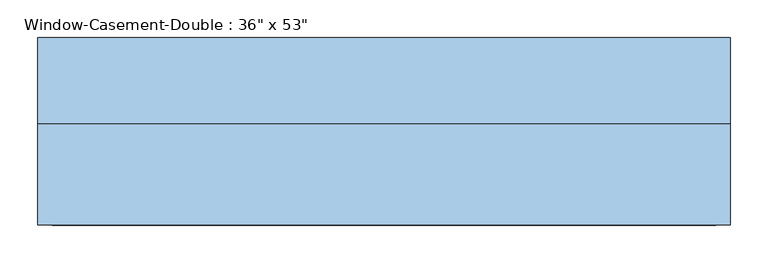
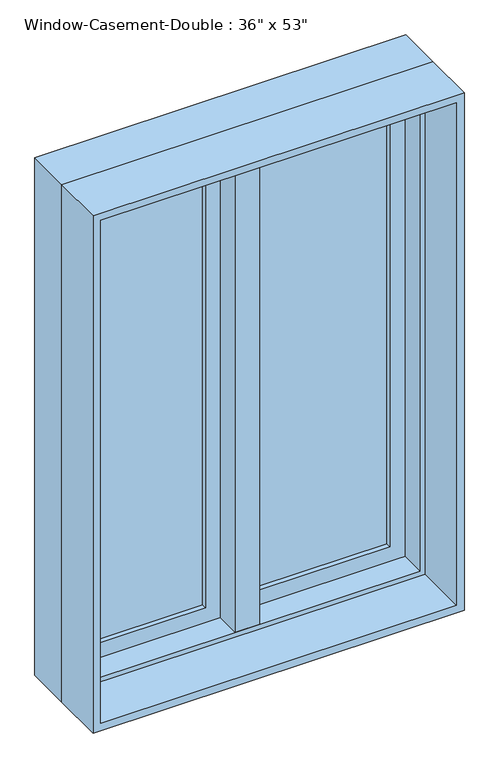
"""IFC4 building model written with IfcOpenShell, lengths in millimetres: window geometry."""

from ifc_helpers import new_model, si_unit, frame, origin, place, context, project, spatial, polyline, outline, extrude, faceted_brep, source, transform, mapped, element, save


def window_79f73a1a(model_context):
    return source(origin(), model_context, "Body", "SolidModel", [
        faceted_brep([(9.525, 133.35, 2247.9), (-9.525, 133.35, 2247.9), (-9.525, 82.55, 2247.9), (9.525, 82.55, 2247.9), (9.525, 133.35, 927.1), (9.525, 82.55, 927.1), (-9.525, 82.55, 927.1), (-9.525, 133.35, 927.1), (-9.525, 82.55, 946.15), (-9.525, 82.55, 2228.85), (-30.1625, 82.55, 946.15), (-30.1625, 82.55, 2228.85), (-30.1625, 19.05, 946.15), (-30.1625, 19.05, 2228.85), (30.1625, 19.05, 946.15), (30.1625, 19.05, 2228.85), (30.1625, 82.55, 946.15), (30.1625, 82.55, 2228.85), (9.525, 82.55, 946.15), (9.525, 82.55, 2228.85)], [[[0, 1, 2, 3]], [[4, 5, 6, 7]], [[1, 0, 4, 7]], [[2, 1, 7, 6, 8, 9]], [[9, 8, 10, 11]], [[11, 10, 12, 13]], [[13, 12, 14, 15]], [[15, 14, 16, 17]], [[17, 16, 18, 19]], [[0, 3, 19, 18, 5, 4]], [[18, 8, 6, 5]], [[9, 19, 3, 2]], [[8, 18, 16, 14, 12, 10]], [[19, 9, 11, 13, 15, 17]]]),
        extrude(outline(polyline([(-66.675, 114.3), (-66.675, 107.95), (-387.35, 107.95), (-387.35, 114.3), (-66.675, 114.3)])), frame((0.0, 0.0, 984.25), z_axis=(0.0, 0.0, 1.0), x_axis=(1.0, 0.0, 0.0)), (0.0, 0.0, 1.0), 1206.5),
        extrude(outline(polyline([(-387.35, 95.25), (-387.35, 101.6), (-66.675, 101.6), (-66.675, 95.25), (-387.35, 95.25)])), frame((0.0, 0.0, 984.25), z_axis=(0.0, 0.0, 1.0), x_axis=(1.0, 0.0, 0.0)), (0.0, 0.0, 1.0), 1206.5),
        extrude(outline(polyline([(387.35, 114.3), (387.35, 107.95), (66.675, 107.95), (66.675, 114.3), (387.35, 114.3)])), frame((0.0, 0.0, 984.25), z_axis=(0.0, 0.0, 1.0), x_axis=(1.0, 0.0, 0.0)), (0.0, 0.0, 1.0), 1206.5),
        extrude(outline(polyline([(66.675, 95.25), (66.675, 101.6), (387.35, 101.6), (387.35, 95.25), (66.675, 95.25)])), frame((0.0, 0.0, 984.25), z_axis=(0.0, 0.0, 1.0), x_axis=(1.0, 0.0, 0.0)), (0.0, 0.0, 1.0), 1206.5),
        extrude(outline(polyline([(2247.9, -444.5), (927.1, -444.5), (927.1, -9.525), (2247.9, -9.525), (2247.9, -444.5)]), holes=[polyline([(2190.75, -66.675), (984.25, -66.675), (984.25, -387.35), (2190.75, -387.35), (2190.75, -66.675)])]), frame((0.0, 82.55, 0.0), z_axis=(0.0, 1.0, 0.0), x_axis=(0.0, 0.0, 1.0)), (0.0, 0.0, 1.0), 44.45),
        extrude(outline(polyline([(927.1, 444.5), (2247.9, 444.5), (2247.9, 9.525), (927.1, 9.525), (927.1, 444.5)]), holes=[polyline([(984.25, 66.675), (2190.75, 66.675), (2190.75, 387.35), (984.25, 387.35), (984.25, 66.675)])]), frame((0.0, 82.55, 0.0), z_axis=(0.0, 1.0, 0.0), x_axis=(0.0, 0.0, 1.0)), (0.0, 0.0, 1.0), 44.45),
        extrude(outline(polyline([(2260.6, -457.2), (914.4, -457.2), (914.4, 457.2), (2260.6, 457.2), (2260.6, -457.2)]), holes=[polyline([(2241.55, 438.15), (933.45, 438.15), (933.45, -438.15), (2241.55, -438.15), (2241.55, 438.15)])]), frame((0.0, -114.3, 0.0), z_axis=(0.0, 1.0, 0.0), x_axis=(0.0, 0.0, 1.0)), (0.0, 0.0, 1.0), 133.35),
        faceted_brep([(425.45, 82.55, 2228.85), (425.45, 19.05, 2228.85), (-425.45, 19.05, 2228.85), (-425.45, 82.55, 2228.85), (444.5, 133.35, 2247.9), (444.5, 82.55, 2247.9), (-444.5, 82.55, 2247.9), (-444.5, 133.35, 2247.9), (457.2, 19.05, 2260.6), (457.2, 133.35, 2260.6), (-457.2, 133.35, 2260.6), (-457.2, 19.05, 2260.6), (-425.45, 19.05, 946.15), (-425.45, 82.55, 946.15), (-444.5, 82.55, 927.1), (-444.5, 133.35, 927.1), (-457.2, 133.35, 914.4), (-457.2, 19.05, 914.4), (425.45, 19.05, 946.15), (425.45, 82.55, 946.15), (444.5, 82.55, 927.1), (444.5, 133.35, 927.1), (457.2, 133.35, 914.4), (457.2, 19.05, 914.4)], [[[0, 1, 2, 3]], [[4, 5, 6, 7]], [[8, 9, 10, 11]], [[3, 2, 12, 13]], [[7, 6, 14, 15]], [[11, 10, 16, 17]], [[13, 12, 18, 19]], [[15, 14, 20, 21]], [[17, 16, 22, 23]], [[11, 17, 23, 8], [1, 18, 12, 2]], [[19, 18, 1, 0]], [[5, 20, 14, 6], [3, 13, 19, 0]], [[21, 20, 5, 4]], [[23, 22, 9, 8]], [[9, 22, 16, 10], [7, 15, 21, 4]]]),
    ])


if __name__ == "__main__":
    model = new_model("IFC4")
    model_context = context("Model", 3, world=origin())
    ifc_project = project(units=[si_unit("LENGTHUNIT", "METRE", prefix="MILLI")], contexts=[model_context])
    site = spatial("IfcSite", under=ifc_project)
    building = spatial("IfcBuilding", under=site)
    placement = place(None, origin())
    window_shape = window_79f73a1a(model_context)
    element("IfcWindow", 1, ObjectType="Window-Casement-Double : 36\" x 53\"", at=placement, inside=building, context=model_context, shape_type="MappedRepresentation", body=[
        mapped(window_shape, transform((0.0, 0.0, 0.0), x_axis=(1.0, 0.0, 0.0), y_axis=(0.0, 1.0, 0.0), z_axis=(0.0, 0.0, 1.0))),
    ])
    save(model, "model.ifc")

# Revit data of these elements
# Type "Window-Casement-Double : 36\" x 53\""
#   Type Mark = "15"
#   Fire Rating = "0.5h"
#   Assembly Code = "B2020100"
#   Analytic Construction = "Double glazing - domestic"
#   Frame Extension [instance default] = 0' - 0 1/4"
#   Window Inset [instance default] = 0' - 0"
#   Wall Thickness [instance default] = 0' - 6"
#   Interior Wall Closure [instance default] = 0' - 2 1/4"
#   Half Width = 1' - 6"
#   Visual Light Transmittance = 0.81
#   Thermal Resistance (R) = 1.8146 (h·ft²·°F)/BTU
#   Solar Heat Gain Coefficient = 0.76
#   Rough Width = 3' - 0 1/2"
#   Rough Height = 4' - 5 1/2"
#   Height = 4' - 5"
#   Heat Transfer Coefficient (U) = 0.5511 BTU/(h·ft²·°F)
#   Exterior Wall Closure [instance default] = 0' - 1 1/4"
#   Extension Jamb [instance default] = 0' - 2 1/4"
#   Default Sill Height = 3' - 0"
#   Width = 3' - 0"
#   Define Thermal Properties by = 0
#   Muntin Visibility = yes
#   Interior Trim Visibility [instance default] = yes
#   Exterior Trim Visibility [instance default] = yes
#   Extension Jamb Visibility [instance default] = yes
#   Interior Trim Material = Wood - Stained
#   Muntin Pattern = Muntin Pattern_2x2 : Muntin Pattern_2x2
#   Interior Trim = Trim-Window-Interior-Flat : Picture Frame
#   Interior Frame Material = Wood - Stained
#   Glass Panel Material = Glass
#   Exterior Trim Material = Clad - White
#   Exterior Trim = Trim-Window-Exterior-Flat : with Sill
#   Exterior Frame Material = Clad - White
#   Wall Closure = (empty or 0)
# Element 1 (IfcWindow, "Window-Casement-Double : 36\" x 53\"")
#   Wall Thickness = 0' - 9"
#   Extension Jamb = 0' - 5 1/4"
#   Materials on its faces: "Wood - Stained", "Glass", "Clad - White"
# Materials
#   "Wood - Stained": class "Wood", colour RGB 224 178 126, transparency 0, Cost = 0
#   "Glass": class "Glass", colour RGB 0 128 192, transparency 0.75, Description = "Soda Lime Glass", Cost = 0
#   "Clad - White": class "Wood", colour RGB 242 242 238, transparency 0, Cost = 0
